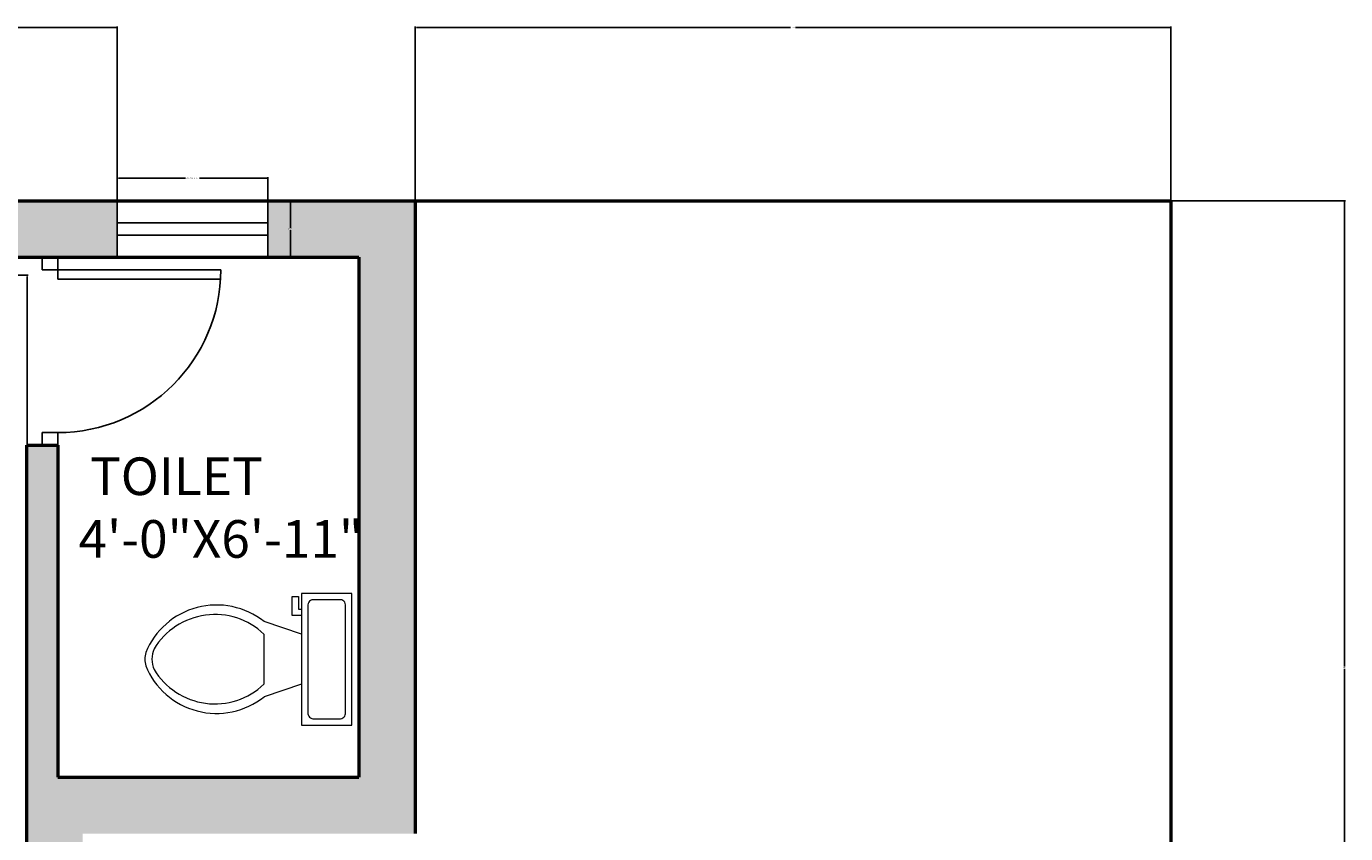
# Model space of a CAD drawing. Units: inches. Extents: x 2831 to 3729, y 3926 to 4974.
# Tile 8 of 8: x 3519 to 3729, y 4845 to 4974. Entities that reach past the tile are written whole.
import ezdxf

# ---------------------------------------------------------------- set-up
doc = ezdxf.new("R2010")
doc.units = ezdxf.units.IN
for name, color, linetype, lineweight in [('A-ANNO-DIMS', 2, 'Continuous', 18), ('A-AREA-IDEN', 7, 'Continuous', 18), ('A-DOOR', 3, 'Continuous', 25), ('A-FLOR-FIXT', 9, 'Continuous', 18), ('A-GLAZ', 4, 'Continuous', 25), ('A-WALL', 7, 'Continuous', 50), ('A-WALL-PATT', 252, 'Continuous', 13)]:
    doc.layers.add(name, color=color, linetype=linetype, lineweight=lineweight)
doc.styles.get("Standard").update_dxf_attribs({"font": 'arial.ttf'})
doc.dimstyles.get("Standard").update_dxf_attribs({"dimtxt": 0.18, "dimasz": 0.18, "dimexe": 0.18, "dimexo": 0.0625, "dimgap": 0.09, "dimtad": 0, "dimtih": 1, "dimtoh": 1, "dimdec": 4, "dimzin": 0, "dimdsep": 46, "dimtxsty": 'Standard', "dimcen": 0.09, "dimadec": 0, "dimazin": 0, "dimtfac": 1, "dimtdec": 4, "dimtofl": 0, "dimtmove": 0, "dimatfit": 3, "dimfxl": 1, "dimtolj": 1, "dimtzin": 0, "dimarcsym": 0})

# ---------------------------------------------------------------- blocks, each defined once
blk = doc.blocks.new('*U8')
for p, q in [((9.5, -6), (9.5, -2)), ((-8, -8.5), (-8, -8)), ((-7, -8), (-7, -9.5)), ((-4, -8), (-6, -14)), ((4, -8), (6, -14)), ((-10, -8.5), (-8, -8.5)), ((-10, -9.5), (-10, -8.5)), ((-7, -9.5), (-10, -9.5)), ((4, -14), (-4, -14))]:
    blk.add_line(p, q)
blk.add_lwpolyline([(10.5, -8), (10.5, 0), (-10.5, 0), (-10.5, -8)], close=True)
for points in [[(-9.5, -2), (-9.5, -6)], [(8.5, -1), (-8.5, -1)], [(-8.5, -7), (8.5, -7)]]:
    blk.add_lwpolyline(points)
for centre, radius, start, end in [((-8.62, -1.88), 0.884, 81.8699, 188.1301), ((8.62, -1.88), 0.884, 351.8699, 98.1301), ((-8.62, -6.12), 0.884, 171.8699, 278.1301), ((8.62, -6.12), 0.884, 261.8699, 8.1301), ((3.52, -21.58), 12.17, 141.4691, 247.9714), ((4.2, -21.82), 11.33, 136.3677, 238.9468), ((-3.52, -21.58), 12.17, 292.0284, 38.5307), ((-4.2, -21.82), 11.33, 301.053, 43.6321), ((0, -27.88), 4, 245.7318, 294.2682), ((0, -29), 4, 254.8605, 285.1395)]:
    blk.add_arc(centre, radius, start, end)
blk = doc.blocks.new('DOOR-SWING-26IN')
for p, q in [((-1.5, 25.96), (-1.5, 0)), ((0, 26), (0, 0)), ((-26, 0), (-28, 0)), ((-26, -2.5), (-26, 0)), ((0, 0), (-1.5, 0)), ((0, -2.5), (0, 0)), ((0, 0), (2, 0)), ((-28, -2.5), (-26, -2.5)), ((2, -2.5), (0, -2.5))]:
    blk.add_line(p, q)
blk.add_arc((0, 0), 26, 90, 180)
blk = doc.blocks.new('WINDOW-24IN-PLAN')
for p, q in [((0, 24), (9, 24)), ((3.5, 0), (3.5, 24)), ((5.5, 0), (5.5, 24)), ((0, 0), (9, 0))]:
    blk.add_line(p, q)
blk = doc.blocks.new('*D25')
at = {"layer": 'A-ANNO-DIMS', "color": 0, "lineweight": -2, "transparency": 16777216}
for p, q in [((3533.31, 4946.2), (3533.31, 4949.92)), ((3533.49, 4949.74), (3544.19, 4949.74)), ((3557.13, 4949.74), (3546.43, 4949.74)), ((3557.31, 4946.2), (3557.31, 4949.92))]:
    blk.add_line(p, q, dxfattribs=at)
at = {"layer": 'A-ANNO-DIMS', "color": 0, "transparency": 16777216}
for points in [[(3533.49, 4949.77), (3533.49, 4949.71), (3533.31, 4949.74)], [(3557.13, 4949.77), (3557.13, 4949.71), (3557.31, 4949.74)]]:
    blk.add_solid(points, dxfattribs=at)
at = {"layer": 'Defpoints', "color": 0, "transparency": 16777216}
for p in [(3557.31, 4949.74), (3533.31, 4946.14), (3557.31, 4946.14)]:
    blk.add_point(p, dxfattribs=at)
at = {"layer": 'A-ANNO-DIMS', "color": 0, "transparency": 16777216, "insert": (3545.31, 4949.74), "char_height": 0.18, "attachment_point": 5}
blk.add_mtext('\\A1;WINDOW 24 TYP.', dxfattribs=at)
blk = doc.blocks.new('*D26')
at = {"layer": 'A-ANNO-DIMS', "color": 0, "lineweight": -2, "transparency": 16777216}
for p, q in [((3557.37, 4946.14), (3561.09, 4946.14)), ((3560.91, 4945.96), (3560.91, 4941.82)), ((3560.91, 4937.32), (3560.91, 4941.46)), ((3557.37, 4937.14), (3561.09, 4937.14))]:
    blk.add_line(p, q, dxfattribs=at)
at = {"layer": 'A-ANNO-DIMS', "color": 0, "transparency": 16777216}
for points in [[(3560.88, 4945.96), (3560.94, 4945.96), (3560.91, 4946.14)], [(3560.88, 4937.32), (3560.94, 4937.32), (3560.91, 4937.14)]]:
    blk.add_solid(points, dxfattribs=at)
at = {"layer": 'Defpoints', "color": 0, "transparency": 16777216}
for p in [(3557.31, 4946.14), (3557.31, 4937.14), (3560.91, 4937.14)]:
    blk.add_point(p, dxfattribs=at)
at = {"layer": 'A-ANNO-DIMS', "color": 0, "transparency": 16777216, "insert": (3560.91, 4941.64), "char_height": 0.18, "attachment_point": 5}
blk.add_mtext('\\A1;9 TYP.', dxfattribs=at)
blk = doc.blocks.new('*D32')
at = {"layer": 'A-ANNO-DIMS', "color": 0, "lineweight": -2, "transparency": 16777216}
for p, q in [((3499.8, 4934.24), (3519.1, 4934.24)), ((3518.92, 4934.06), (3518.92, 4880.81)), ((3518.92, 4827.2), (3518.92, 4880.45)), ((3499.8, 4827.02), (3519.1, 4827.02))]:
    blk.add_line(p, q, dxfattribs=at)
at = {"layer": 'A-ANNO-DIMS', "color": 0, "transparency": 16777216}
for points in [[(3518.89, 4934.06), (3518.95, 4934.06), (3518.92, 4934.24)], [(3518.89, 4827.2), (3518.95, 4827.2), (3518.92, 4827.02)]]:
    blk.add_solid(points, dxfattribs=at)
at = {"layer": 'Defpoints', "color": 0, "transparency": 16777216}
for p in [(3499.74, 4934.24), (3518.92, 4934.24), (3499.74, 4827.02)]:
    blk.add_point(p, dxfattribs=at)
at = {"layer": 'A-ANNO-DIMS', "color": 0, "transparency": 16777216, "insert": (3518.92, 4880.63), "char_height": 0.18, "attachment_point": 5}
blk.add_mtext('\\A1;107', dxfattribs=at)
blk = doc.blocks.new('*D56')
at = {"layer": 'A-ANNO-DIMS', "color": 0, "lineweight": -2, "transparency": 16777216}
for p, q in [((3580.81, 4946.2), (3580.81, 4973.97)), ((3580.99, 4973.79), (3640.67, 4973.79)), ((3701.13, 4973.79), (3641.44, 4973.79)), ((3701.31, 4946.2), (3701.31, 4973.97))]:
    blk.add_line(p, q, dxfattribs=at)
at = {"layer": 'A-ANNO-DIMS', "color": 0, "transparency": 16777216}
for points in [[(3580.99, 4973.82), (3580.99, 4973.76), (3580.81, 4973.79)], [(3701.13, 4973.82), (3701.13, 4973.76), (3701.31, 4973.79)]]:
    blk.add_solid(points, dxfattribs=at)
at = {"layer": 'Defpoints', "color": 0, "transparency": 16777216}
for p in [(3701.31, 4973.79), (3580.81, 4946.14), (3701.31, 4946.14)]:
    blk.add_point(p, dxfattribs=at)
at = {"layer": 'A-ANNO-DIMS', "color": 0, "transparency": 16777216, "insert": (3641.06, 4973.79), "char_height": 0.18, "attachment_point": 5}
blk.add_mtext('\\A1;120.5', dxfattribs=at)
blk = doc.blocks.new('*D57')
at = {"layer": 'A-ANNO-DIMS', "color": 0, "lineweight": -2, "transparency": 16777216}
for p, q in [((3701.37, 4946.14), (3729.14, 4946.14)), ((3728.96, 4945.96), (3728.96, 4871.82)), ((3728.96, 4797.32), (3728.96, 4871.46)), ((3701.37, 4797.14), (3729.14, 4797.14))]:
    blk.add_line(p, q, dxfattribs=at)
at = {"layer": 'A-ANNO-DIMS', "color": 0, "transparency": 16777216}
for points in [[(3728.93, 4945.96), (3728.99, 4945.96), (3728.96, 4946.14)], [(3728.93, 4797.32), (3728.99, 4797.32), (3728.96, 4797.14)]]:
    blk.add_solid(points, dxfattribs=at)
at = {"layer": 'Defpoints', "color": 0, "transparency": 16777216}
for p in [(3701.31, 4946.14), (3728.96, 4946.14), (3701.31, 4797.14)]:
    blk.add_point(p, dxfattribs=at)
at = {"layer": 'A-ANNO-DIMS', "color": 0, "transparency": 16777216, "insert": (3728.96, 4871.64), "char_height": 0.18, "attachment_point": 5}
blk.add_mtext('\\A1;149', dxfattribs=at)
blk = doc.blocks.new('*D58')
at = {"layer": 'A-ANNO-DIMS', "color": 0, "lineweight": -2, "transparency": 16777216}
for p, q in [((3470.56, 4946.2), (3470.56, 4973.97)), ((3470.74, 4973.79), (3501.54, 4973.79)), ((3533.13, 4973.79), (3502.33, 4973.79)), ((3533.31, 4946.2), (3533.31, 4973.97))]:
    blk.add_line(p, q, dxfattribs=at)
at = {"layer": 'A-ANNO-DIMS', "color": 0, "transparency": 16777216}
for points in [[(3470.74, 4973.82), (3470.74, 4973.76), (3470.56, 4973.79)], [(3533.13, 4973.82), (3533.13, 4973.76), (3533.31, 4973.79)]]:
    blk.add_solid(points, dxfattribs=at)
at = {"layer": 'Defpoints', "color": 0, "transparency": 16777216}
for p in [(3533.31, 4973.79), (3470.56, 4946.14), (3533.31, 4946.14)]:
    blk.add_point(p, dxfattribs=at)
at = {"layer": 'A-ANNO-DIMS', "color": 0, "transparency": 16777216, "insert": (3501.93, 4973.79), "char_height": 0.18, "attachment_point": 5}
blk.add_mtext('\\A1;62.75', dxfattribs=at)

msp = doc.modelspace()

# ---------------------------------------------------------------- hatches: boundary and pattern name
at = {"layer": 'A-WALL-PATT'}
h = msp.add_hatch(color=256, dxfattribs=at)
h.dxf.hatch_style = 1
h.paths.add_polyline_path([(3533.3091, 4946.1405), (3470.5591, 4946.1405), (3470.5591, 4937.1405), (3518.8091, 4937.1405), (3533.3091, 4937.1405)])
h = msp.add_hatch(color=256, dxfattribs=at)
h.dxf.hatch_style = 1
h.paths.add_polyline_path([(3580.8091, 4946.1405), (3557.3091, 4946.1405), (3557.3091, 4937.1405), (3571.8091, 4937.1405), (3571.8091, 4854.1405), (3523.8091, 4854.1405), (3523.8091, 4907.1405), (3518.8091, 4907.1405), (3518.8091, 4788.1405), (3527.8091, 4788.1405), (3527.8091, 4845.1405), (3580.8091, 4845.1405)])

# ---------------------------------------------------------------- linework, layer by layer
at = {"layer": 'A-WALL'}
for p, q in [((3341.3091, 4946.1405), (3701.3091, 4946.1405)), ((3580.8091, 4946.1405), (3580.8091, 4845.1405)), ((3701.3091, 4946.1405), (3701.3091, 4466.1405)), ((3350.3091, 4937.1405), (3518.8091, 4937.1405)), ((3518.8091, 4937.1405), (3571.8091, 4937.1405)), ((3571.8091, 4937.1405), (3571.8091, 4854.1405)), ((3518.8091, 4907.1405), (3518.8091, 4788.1405)), ((3518.8091, 4907.1405), (3523.8091, 4907.1405)), ((3523.8091, 4907.1405), (3523.8091, 4854.1405)), ((3523.8091, 4854.1405), (3571.8091, 4854.1405))]:
    msp.add_line(p, q, dxfattribs=at)

# ---------------------------------------------------------------- block references
at = {"layer": 'A-DOOR', "extrusion": (0, 0, -1), "zscale": -1, "rotation": 90.00000000000433}
msp.add_blockref('DOOR-SWING-26IN', (-3523.8091, 4935.1405), dxfattribs=at)
at = {"layer": 'A-FLOR-FIXT', "rotation": 270}
msp.add_blockref('*U8', (3570.6983, 4872.9774), dxfattribs=at)
at = {"layer": 'A-GLAZ', "rotation": 270.0000000000045}
msp.add_blockref('WINDOW-24IN-PLAN', (3533.3091, 4946.1405), dxfattribs=at)

# ---------------------------------------------------------------- texts
at = {"layer": 'A-AREA-IDEN', "insert": (3527.1218, 4905.1719), "char_height": 6, "attachment_point": 1}
msp.add_mtext_dynamic_manual_height_columns(' TOILET\\P4\'-0"X6\'-11"', width=76.299971, gutter_width=12.5, heights=[0], dxfattribs=at)

# ---------------------------------------------------------------- dimensions: what is measured, and where the dimension line sits
at = {"layer": 'A-ANNO-DIMS'}
for base, p1, p2, override, picture, middle in [((3533.3091, 4973.7905), (3470.5591, 4946.1405), (3533.3091, 4946.1405), {"dimdec": 2, "dimlfac": 1, "dimrnd": 0, "dimzin": 0, "dimdsep": 46, "dimlunit": 2}, '*D58', (3501.9341, 4973.7905)), ((3701.3091, 4973.7905), (3580.8091, 4946.1405), (3701.3091, 4946.1405), {"dimdec": 1, "dimlfac": 1, "dimrnd": 0, "dimzin": 0, "dimdsep": 46, "dimlunit": 2}, '*D56', (3641.0591, 4973.7905))]:
    dim = msp.add_linear_dim(base=base, p1=p1, p2=p2, dimstyle='Standard', override=override, dxfattribs=at)
    dim.commit()
    dim.dimension.update_dxf_attribs({"geometry": picture, "text_midpoint": middle})
for base, p1, p2, angle, text, picture, middle in [((3557.3091, 4949.7405), (3533.3091, 4946.1405), (3557.3091, 4946.1405), 0, 'WINDOW <> TYP.', '*D25', (3545.3091, 4949.7405)), ((3560.9091, 4937.1405), (3557.3091, 4946.1405), (3557.3091, 4937.1405), 270, '<> TYP.', '*D26', (3560.9091, 4941.6405))]:
    dim = msp.add_linear_dim(base=base, p1=p1, p2=p2, angle=angle, text=text, dimstyle='Standard', override={"dimdec": 0, "dimlfac": 1, "dimrnd": 0, "dimzin": 0, "dimdsep": 46, "dimlunit": 2}, dxfattribs=at)
    dim.commit()
    dim.dimension.update_dxf_attribs({"geometry": picture, "text_midpoint": middle})
for base, p1, p2, picture, middle in [((3728.9591, 4946.1405), (3701.3091, 4797.1405), (3701.3091, 4946.1405), '*D57', (3728.9591, 4871.6405)), ((3518.9199, 4934.242), (3499.7423, 4827.0157), (3499.7423, 4934.242), '*D32', (3518.9199, 4880.6288))]:
    dim = msp.add_linear_dim(base=base, p1=p1, p2=p2, angle=90, dimstyle='Standard', override={"dimdec": 0, "dimlfac": 1, "dimrnd": 0, "dimzin": 0, "dimdsep": 46, "dimlunit": 2}, dxfattribs=at)
    dim.commit()
    dim.dimension.update_dxf_attribs({"geometry": picture, "text_midpoint": middle})

doc.saveas('drawing.dxf')
